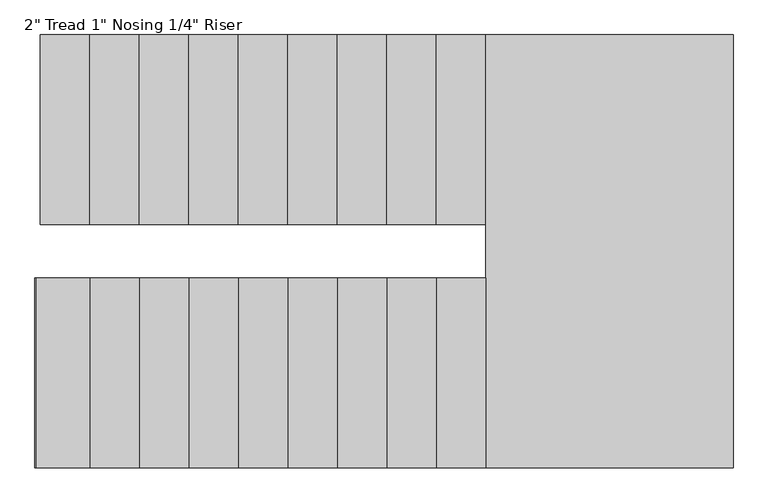
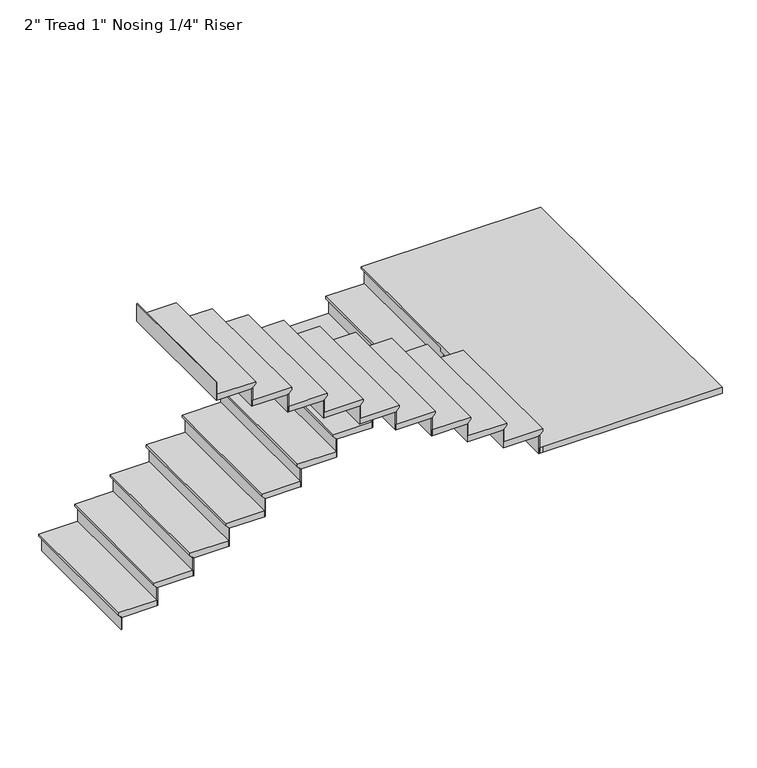
"""IFC4 building model written with IfcOpenShell, lengths in millimetres: stair flight geometry."""

from ifc_helpers import new_model, si_unit, origin, place, context, project, spatial, faceted_brep, source, transform, mapped, element, save


def stair_flight_54cbe99c(model_context):
    return source(origin(), model_context, "Body", "Brep", [
        faceted_brep([(9166.2546318, 21751.034892, 140.97), (9166.2546318, 21751.034892, 160.02), (9166.2546318, 22919.434892, 160.02), (9166.2546318, 22919.434892, 140.97), (9191.6546318, 21751.034892, 115.57), (9191.6546318, 22919.434892, 115.57), (9496.4546318, 21751.034892, 160.02), (9496.4546318, 22919.434892, 160.02), (9191.6546318, 22919.434892, 109.22), (9496.4546318, 22919.434892, 109.22), (9496.4546318, 21751.034892, 109.22), (9191.6546318, 21751.034892, 109.22)], [[[0, 1, 2, 3]], [[4, 0, 3, 5]], [[2, 1, 6, 7]], [[8, 9, 10, 11]], [[2, 7, 9, 8, 5, 3]], [[8, 11, 4, 5]], [[6, 1, 0, 4, 11, 10]], [[7, 6, 10, 9]]]),
        faceted_brep([(9191.6546318, 21751.034892, 109.22), (9191.6546318, 21751.034892, 0.0), (9198.0046318, 21751.034892, 0.0), (9198.0046318, 21751.034892, 109.22), (9191.6546318, 22919.434892, 109.22), (9198.0046318, 22919.434892, 109.22), (9198.0046318, 22919.434892, 0.0), (9191.6546318, 22919.434892, 0.0)], [[[0, 1, 2, 3]], [[4, 5, 6, 7]], [[1, 0, 4, 7]], [[2, 1, 7, 6]], [[3, 2, 6, 5]], [[0, 3, 5, 4]]]),
        faceted_brep([(9496.4546318, 21751.034892, 269.24), (9496.4546318, 21751.034892, 109.22), (9502.8046318, 21751.034892, 109.22), (9502.8046318, 21751.034892, 269.24), (9496.4546318, 22919.434892, 269.24), (9502.8046318, 22919.434892, 269.24), (9502.8046318, 22919.434892, 109.22), (9496.4546318, 22919.434892, 109.22)], [[[0, 1, 2, 3]], [[4, 5, 6, 7]], [[1, 0, 4, 7]], [[2, 1, 7, 6]], [[3, 2, 6, 5]], [[0, 3, 5, 4]]]),
        faceted_brep([(9471.0546318, 22919.434892, 320.04), (9471.0546318, 21751.034892, 320.04), (9801.2546318, 21751.034892, 320.04), (9801.2546318, 22919.434892, 320.04), (9496.4546318, 22919.434892, 269.24), (9801.2546318, 22919.434892, 269.24), (9801.2546318, 21751.034892, 269.24), (9496.4546318, 21751.034892, 269.24), (9496.4546318, 22919.434892, 275.59), (9471.0546318, 22919.434892, 300.99), (9496.4546318, 21751.034892, 275.59), (9471.0546318, 21751.034892, 300.99)], [[[0, 1, 2, 3]], [[4, 5, 6, 7]], [[0, 3, 5, 4, 8, 9]], [[4, 7, 10, 8]], [[2, 1, 11, 10, 7, 6]], [[3, 2, 6, 5]], [[11, 1, 0, 9]], [[10, 11, 9, 8]]]),
        faceted_brep([(9801.2546318, 21751.034892, 429.26), (9801.2546318, 21751.034892, 269.24), (9807.6046318, 21751.034892, 269.24), (9807.6046318, 21751.034892, 429.26), (9801.2546318, 22919.434892, 429.26), (9807.6046318, 22919.434892, 429.26), (9807.6046318, 22919.434892, 269.24), (9801.2546318, 22919.434892, 269.24)], [[[0, 1, 2, 3]], [[4, 5, 6, 7]], [[1, 0, 4, 7]], [[2, 1, 7, 6]], [[3, 2, 6, 5]], [[0, 3, 5, 4]]]),
        faceted_brep([(9775.8546318, 22919.434892, 480.06), (9775.8546318, 21751.034892, 480.06), (10106.0546318, 21751.034892, 480.06), (10106.0546318, 22919.434892, 480.06), (9801.2546318, 22919.434892, 429.26), (10106.0546318, 22919.434892, 429.26), (10106.0546318, 21751.034892, 429.26), (9801.2546318, 21751.034892, 429.26), (9801.2546318, 22919.434892, 435.61), (9775.8546318, 22919.434892, 461.01), (9801.2546318, 21751.034892, 435.61), (9775.8546318, 21751.034892, 461.01)], [[[0, 1, 2, 3]], [[4, 5, 6, 7]], [[0, 3, 5, 4, 8, 9]], [[4, 7, 10, 8]], [[2, 1, 11, 10, 7, 6]], [[3, 2, 6, 5]], [[11, 1, 0, 9]], [[10, 11, 9, 8]]]),
        faceted_brep([(10106.0546318, 21751.034892, 589.28), (10106.0546318, 21751.034892, 429.26), (10112.4046318, 21751.034892, 429.26), (10112.4046318, 21751.034892, 589.28), (10106.0546318, 22919.434892, 589.28), (10112.4046318, 22919.434892, 589.28), (10112.4046318, 22919.434892, 429.26), (10106.0546318, 22919.434892, 429.26)], [[[0, 1, 2, 3]], [[4, 5, 6, 7]], [[1, 0, 4, 7]], [[2, 1, 7, 6]], [[3, 2, 6, 5]], [[0, 3, 5, 4]]]),
        faceted_brep([(10080.6546318, 22919.434892, 640.08), (10080.6546318, 21751.034892, 640.08), (10410.8546318, 21751.034892, 640.08), (10410.8546318, 22919.434892, 640.08), (10106.0546318, 22919.434892, 589.28), (10410.8546318, 22919.434892, 589.28), (10410.8546318, 21751.034892, 589.28), (10106.0546318, 21751.034892, 589.28), (10106.0546318, 22919.434892, 595.63), (10080.6546318, 22919.434892, 621.03), (10106.0546318, 21751.034892, 595.63), (10080.6546318, 21751.034892, 621.03)], [[[0, 1, 2, 3]], [[4, 5, 6, 7]], [[0, 3, 5, 4, 8, 9]], [[4, 7, 10, 8]], [[2, 1, 11, 10, 7, 6]], [[3, 2, 6, 5]], [[11, 1, 0, 9]], [[10, 11, 9, 8]]]),
        faceted_brep([(10410.8546318, 21751.034892, 749.3), (10410.8546318, 21751.034892, 589.28), (10417.2046318, 21751.034892, 589.28), (10417.2046318, 21751.034892, 749.3), (10410.8546318, 22919.434892, 749.3), (10417.2046318, 22919.434892, 749.3), (10417.2046318, 22919.434892, 589.28), (10410.8546318, 22919.434892, 589.28)], [[[0, 1, 2, 3]], [[4, 5, 6, 7]], [[1, 0, 4, 7]], [[2, 1, 7, 6]], [[3, 2, 6, 5]], [[0, 3, 5, 4]]]),
        faceted_brep([(10385.4546318, 22919.434892, 800.1), (10385.4546318, 21751.034892, 800.1), (10715.6546318, 21751.034892, 800.1), (10715.6546318, 22919.434892, 800.1), (10410.8546318, 22919.434892, 749.3), (10715.6546318, 22919.434892, 749.3), (10715.6546318, 21751.034892, 749.3), (10410.8546318, 21751.034892, 749.3), (10410.8546318, 22919.434892, 755.65), (10385.4546318, 22919.434892, 781.05), (10410.8546318, 21751.034892, 755.65), (10385.4546318, 21751.034892, 781.05)], [[[0, 1, 2, 3]], [[4, 5, 6, 7]], [[0, 3, 5, 4, 8, 9]], [[4, 7, 10, 8]], [[2, 1, 11, 10, 7, 6]], [[3, 2, 6, 5]], [[11, 1, 0, 9]], [[10, 11, 9, 8]]]),
        faceted_brep([(10715.6546318, 21751.034892, 909.32), (10715.6546318, 21751.034892, 749.3), (10722.0046318, 21751.034892, 749.3), (10722.0046318, 21751.034892, 909.32), (10715.6546318, 22919.434892, 909.32), (10722.0046318, 22919.434892, 909.32), (10722.0046318, 22919.434892, 749.3), (10715.6546318, 22919.434892, 749.3)], [[[0, 1, 2, 3]], [[4, 5, 6, 7]], [[1, 0, 4, 7]], [[2, 1, 7, 6]], [[3, 2, 6, 5]], [[0, 3, 5, 4]]]),
        faceted_brep([(10690.2546318, 22919.434892, 960.12), (10690.2546318, 21751.034892, 960.12), (11020.4546318, 21751.034892, 960.12), (11020.4546318, 22919.434892, 960.12), (10715.6546318, 22919.434892, 909.32), (11020.4546318, 22919.434892, 909.32), (11020.4546318, 21751.034892, 909.32), (10715.6546318, 21751.034892, 909.32), (10715.6546318, 22919.434892, 915.67), (10690.2546318, 22919.434892, 941.07), (10715.6546318, 21751.034892, 915.67), (10690.2546318, 21751.034892, 941.07)], [[[0, 1, 2, 3]], [[4, 5, 6, 7]], [[0, 3, 5, 4, 8, 9]], [[4, 7, 10, 8]], [[2, 1, 11, 10, 7, 6]], [[3, 2, 6, 5]], [[11, 1, 0, 9]], [[10, 11, 9, 8]]]),
        faceted_brep([(11020.4546318, 21751.034892, 1069.34), (11020.4546318, 21751.034892, 909.32), (11026.8046318, 21751.034892, 909.32), (11026.8046318, 21751.034892, 1069.34), (11020.4546318, 22919.434892, 1069.34), (11026.8046318, 22919.434892, 1069.34), (11026.8046318, 22919.434892, 909.32), (11020.4546318, 22919.434892, 909.32)], [[[0, 1, 2, 3]], [[4, 5, 6, 7]], [[1, 0, 4, 7]], [[2, 1, 7, 6]], [[3, 2, 6, 5]], [[0, 3, 5, 4]]]),
        faceted_brep([(10995.0546318, 22919.434892, 1120.14), (10995.0546318, 21751.034892, 1120.14), (11325.2546318, 21751.034892, 1120.14), (11325.2546318, 22919.434892, 1120.14), (11020.4546318, 22919.434892, 1069.34), (11325.2546318, 22919.434892, 1069.34), (11325.2546318, 21751.034892, 1069.34), (11020.4546318, 21751.034892, 1069.34), (11020.4546318, 22919.434892, 1075.69), (10995.0546318, 22919.434892, 1101.09), (11020.4546318, 21751.034892, 1075.69), (10995.0546318, 21751.034892, 1101.09)], [[[0, 1, 2, 3]], [[4, 5, 6, 7]], [[0, 3, 5, 4, 8, 9]], [[4, 7, 10, 8]], [[2, 1, 11, 10, 7, 6]], [[3, 2, 6, 5]], [[11, 1, 0, 9]], [[10, 11, 9, 8]]]),
        faceted_brep([(11325.2546318, 21751.034892, 1229.36), (11325.2546318, 21751.034892, 1069.34), (11331.6046318, 21751.034892, 1069.34), (11331.6046318, 21751.034892, 1229.36), (11325.2546318, 22919.434892, 1229.36), (11331.6046318, 22919.434892, 1229.36), (11331.6046318, 22919.434892, 1069.34), (11325.2546318, 22919.434892, 1069.34)], [[[0, 1, 2, 3]], [[4, 5, 6, 7]], [[1, 0, 4, 7]], [[2, 1, 7, 6]], [[3, 2, 6, 5]], [[0, 3, 5, 4]]]),
        faceted_brep([(11299.8546318, 22919.434892, 1280.16), (11299.8546318, 21751.034892, 1280.16), (11630.0546318, 21751.034892, 1280.16), (11630.0546318, 22919.434892, 1280.16), (11325.2546318, 22919.434892, 1229.36), (11630.0546318, 22919.434892, 1229.36), (11630.0546318, 21751.034892, 1229.36), (11325.2546318, 21751.034892, 1229.36), (11325.2546318, 22919.434892, 1235.71), (11299.8546318, 22919.434892, 1261.11), (11325.2546318, 21751.034892, 1235.71), (11299.8546318, 21751.034892, 1261.11)], [[[0, 1, 2, 3]], [[4, 5, 6, 7]], [[0, 3, 5, 4, 8, 9]], [[4, 7, 10, 8]], [[2, 1, 11, 10, 7, 6]], [[3, 2, 6, 5]], [[11, 1, 0, 9]], [[10, 11, 9, 8]]]),
        faceted_brep([(11630.0546318, 21751.034892, 1389.38), (11630.0546318, 21751.034892, 1229.36), (11636.4046318, 21751.034892, 1229.36), (11636.4046318, 21751.034892, 1389.38), (11630.0546318, 22919.434892, 1389.38), (11636.4046318, 22919.434892, 1389.38), (11636.4046318, 22919.434892, 1229.36), (11630.0546318, 22919.434892, 1229.36)], [[[0, 1, 2, 3]], [[4, 5, 6, 7]], [[1, 0, 4, 7]], [[2, 1, 7, 6]], [[3, 2, 6, 5]], [[0, 3, 5, 4]]]),
        faceted_brep([(11604.6546318, 22919.434892, 1440.18), (11604.6546318, 21751.034892, 1440.18), (11934.8546318, 21751.034892, 1440.18), (11934.8546318, 22919.434892, 1440.18), (11630.0546318, 22919.434892, 1389.38), (11934.8546318, 22919.434892, 1389.38), (11934.8546318, 21751.034892, 1389.38), (11630.0546318, 21751.034892, 1389.38), (11630.0546318, 22919.434892, 1395.73), (11604.6546318, 22919.434892, 1421.13), (11630.0546318, 21751.034892, 1395.73), (11604.6546318, 21751.034892, 1421.13)], [[[0, 1, 2, 3]], [[4, 5, 6, 7]], [[0, 3, 5, 4, 8, 9]], [[4, 7, 10, 8]], [[2, 1, 11, 10, 7, 6]], [[3, 2, 6, 5]], [[11, 1, 0, 9]], [[10, 11, 9, 8]]]),
        faceted_brep([(11934.8546318, 21751.034892, 1549.4), (11934.8546318, 21751.034892, 1389.38), (11941.2046318, 21751.034892, 1389.38), (11941.2046318, 21751.034892, 1549.4), (11934.8546318, 22919.434892, 1549.4), (11941.2046318, 22919.434892, 1549.4), (11941.2046318, 22919.434892, 1389.38), (11934.8546318, 22919.434892, 1389.38)], [[[0, 1, 2, 3]], [[4, 5, 6, 7]], [[1, 0, 4, 7]], [[2, 1, 7, 6]], [[3, 2, 6, 5]], [[0, 3, 5, 4]]]),
        faceted_brep([(11884.0546318, 20252.434892, 1600.2), (11909.4546318, 20252.434892, 1600.2), (13433.4546318, 20252.434892, 1600.2), (13433.4546318, 22919.434892, 1600.2), (11909.4546318, 22919.434892, 1600.2), (11909.4546318, 21420.834892, 1600.2), (11884.0546318, 21420.834892, 1600.2), (11909.4546318, 20252.434892, 1549.4), (11884.0546318, 20252.434892, 1549.4), (11884.0546318, 21420.834892, 1549.4), (11909.4546318, 21420.834892, 1549.4), (11909.4546318, 21751.034892, 1549.4), (11934.8546318, 21751.034892, 1549.4), (11934.8546318, 22919.434892, 1549.4), (13433.4546318, 22919.434892, 1549.4), (13433.4546318, 20252.434892, 1549.4), (11934.8546318, 22919.434892, 1555.75), (11909.4546318, 22919.434892, 1581.15), (11934.8546318, 21751.034892, 1555.75), (11909.4546318, 21751.034892, 1581.15)], [[[0, 1, 2, 3, 4, 5, 6]], [[7, 8, 9, 10, 11, 12, 13, 14, 15]], [[1, 0, 8, 7]], [[2, 1, 7, 15]], [[3, 2, 15, 14]], [[4, 3, 14, 13, 16, 17]], [[13, 12, 18, 16]], [[12, 11, 19, 18]], [[5, 4, 17, 19, 11, 10]], [[6, 5, 10, 9]], [[0, 6, 9, 8]], [[17, 16, 18, 19]]]),
        faceted_brep([(11884.0546318, 21420.834892, 1709.42), (11884.0546318, 21420.834892, 1549.4), (11877.7046318, 21420.834892, 1549.4), (11877.7046318, 21420.834892, 1709.42), (11884.0546318, 20252.434892, 1709.42), (11877.7046318, 20252.434892, 1709.42), (11877.7046318, 20252.434892, 1549.4), (11884.0546318, 20252.434892, 1549.4)], [[[0, 1, 2, 3]], [[4, 5, 6, 7]], [[1, 0, 4, 7]], [[2, 1, 7, 6]], [[3, 2, 6, 5]], [[0, 3, 5, 4]]]),
        faceted_brep([(11909.4546318, 20252.434892, 1760.22), (11909.4546318, 21420.834892, 1760.22), (11579.2546318, 21420.834892, 1760.22), (11579.2546318, 20252.434892, 1760.22), (11884.0546318, 20252.434892, 1709.42), (11579.2546318, 20252.434892, 1709.42), (11579.2546318, 21420.834892, 1709.42), (11884.0546318, 21420.834892, 1709.42), (11884.0546318, 20252.434892, 1715.77), (11909.4546318, 20252.434892, 1741.17), (11884.0546318, 21420.834892, 1715.77), (11909.4546318, 21420.834892, 1741.17)], [[[0, 1, 2, 3]], [[4, 5, 6, 7]], [[0, 3, 5, 4, 8, 9]], [[4, 7, 10, 8]], [[2, 1, 11, 10, 7, 6]], [[3, 2, 6, 5]], [[11, 1, 0, 9]], [[10, 11, 9, 8]]]),
        faceted_brep([(11579.2546318, 21420.834892, 1869.44), (11579.2546318, 21420.834892, 1709.42), (11572.9046318, 21420.834892, 1709.42), (11572.9046318, 21420.834892, 1869.44), (11579.2546318, 20252.434892, 1869.44), (11572.9046318, 20252.434892, 1869.44), (11572.9046318, 20252.434892, 1709.42), (11579.2546318, 20252.434892, 1709.42)], [[[0, 1, 2, 3]], [[4, 5, 6, 7]], [[1, 0, 4, 7]], [[2, 1, 7, 6]], [[3, 2, 6, 5]], [[0, 3, 5, 4]]]),
        faceted_brep([(11604.6546318, 20252.434892, 1920.24), (11604.6546318, 21420.834892, 1920.24), (11274.4546318, 21420.834892, 1920.24), (11274.4546318, 20252.434892, 1920.24), (11579.2546318, 20252.434892, 1869.44), (11274.4546318, 20252.434892, 1869.44), (11274.4546318, 21420.834892, 1869.44), (11579.2546318, 21420.834892, 1869.44), (11579.2546318, 20252.434892, 1875.79), (11604.6546318, 20252.434892, 1901.19), (11579.2546318, 21420.834892, 1875.79), (11604.6546318, 21420.834892, 1901.19)], [[[0, 1, 2, 3]], [[4, 5, 6, 7]], [[0, 3, 5, 4, 8, 9]], [[4, 7, 10, 8]], [[2, 1, 11, 10, 7, 6]], [[3, 2, 6, 5]], [[11, 1, 0, 9]], [[10, 11, 9, 8]]]),
        faceted_brep([(11274.4546318, 21420.834892, 2029.46), (11274.4546318, 21420.834892, 1869.44), (11268.1046318, 21420.834892, 1869.44), (11268.1046318, 21420.834892, 2029.46), (11274.4546318, 20252.434892, 2029.46), (11268.1046318, 20252.434892, 2029.46), (11268.1046318, 20252.434892, 1869.44), (11274.4546318, 20252.434892, 1869.44)], [[[0, 1, 2, 3]], [[4, 5, 6, 7]], [[1, 0, 4, 7]], [[2, 1, 7, 6]], [[3, 2, 6, 5]], [[0, 3, 5, 4]]]),
        faceted_brep([(11299.8546318, 20252.434892, 2080.26), (11299.8546318, 21420.834892, 2080.26), (10969.6546318, 21420.834892, 2080.26), (10969.6546318, 20252.434892, 2080.26), (11274.4546318, 20252.434892, 2029.46), (10969.6546318, 20252.434892, 2029.46), (10969.6546318, 21420.834892, 2029.46), (11274.4546318, 21420.834892, 2029.46), (11274.4546318, 20252.434892, 2035.81), (11299.8546318, 20252.434892, 2061.21), (11274.4546318, 21420.834892, 2035.81), (11299.8546318, 21420.834892, 2061.21)], [[[0, 1, 2, 3]], [[4, 5, 6, 7]], [[0, 3, 5, 4, 8, 9]], [[4, 7, 10, 8]], [[2, 1, 11, 10, 7, 6]], [[3, 2, 6, 5]], [[11, 1, 0, 9]], [[10, 11, 9, 8]]]),
        faceted_brep([(10969.6546318, 21420.834892, 2189.48), (10969.6546318, 21420.834892, 2029.46), (10963.3046318, 21420.834892, 2029.46), (10963.3046318, 21420.834892, 2189.48), (10969.6546318, 20252.434892, 2189.48), (10963.3046318, 20252.434892, 2189.48), (10963.3046318, 20252.434892, 2029.46), (10969.6546318, 20252.434892, 2029.46)], [[[0, 1, 2, 3]], [[4, 5, 6, 7]], [[1, 0, 4, 7]], [[2, 1, 7, 6]], [[3, 2, 6, 5]], [[0, 3, 5, 4]]]),
        faceted_brep([(10995.0546318, 20252.434892, 2240.28), (10995.0546318, 21420.834892, 2240.28), (10664.8546318, 21420.834892, 2240.28), (10664.8546318, 20252.434892, 2240.28), (10969.6546318, 20252.434892, 2189.48), (10664.8546318, 20252.434892, 2189.48), (10664.8546318, 21420.834892, 2189.48), (10969.6546318, 21420.834892, 2189.48), (10969.6546318, 20252.434892, 2195.83), (10995.0546318, 20252.434892, 2221.23), (10969.6546318, 21420.834892, 2195.83), (10995.0546318, 21420.834892, 2221.23)], [[[0, 1, 2, 3]], [[4, 5, 6, 7]], [[0, 3, 5, 4, 8, 9]], [[4, 7, 10, 8]], [[2, 1, 11, 10, 7, 6]], [[3, 2, 6, 5]], [[11, 1, 0, 9]], [[10, 11, 9, 8]]]),
        faceted_brep([(10664.8546318, 21420.834892, 2349.5), (10664.8546318, 21420.834892, 2189.48), (10658.5046318, 21420.834892, 2189.48), (10658.5046318, 21420.834892, 2349.5), (10664.8546318, 20252.434892, 2349.5), (10658.5046318, 20252.434892, 2349.5), (10658.5046318, 20252.434892, 2189.48), (10664.8546318, 20252.434892, 2189.48)], [[[0, 1, 2, 3]], [[4, 5, 6, 7]], [[1, 0, 4, 7]], [[2, 1, 7, 6]], [[3, 2, 6, 5]], [[0, 3, 5, 4]]]),
        faceted_brep([(10690.2546318, 20252.434892, 2400.3), (10690.2546318, 21420.834892, 2400.3), (10360.0546318, 21420.834892, 2400.3), (10360.0546318, 20252.434892, 2400.3), (10664.8546318, 20252.434892, 2349.5), (10360.0546318, 20252.434892, 2349.5), (10360.0546318, 21420.834892, 2349.5), (10664.8546318, 21420.834892, 2349.5), (10664.8546318, 20252.434892, 2355.85), (10690.2546318, 20252.434892, 2381.25), (10664.8546318, 21420.834892, 2355.85), (10690.2546318, 21420.834892, 2381.25)], [[[0, 1, 2, 3]], [[4, 5, 6, 7]], [[0, 3, 5, 4, 8, 9]], [[4, 7, 10, 8]], [[2, 1, 11, 10, 7, 6]], [[3, 2, 6, 5]], [[11, 1, 0, 9]], [[10, 11, 9, 8]]]),
        faceted_brep([(10360.0546318, 21420.834892, 2509.52), (10360.0546318, 21420.834892, 2349.5), (10353.7046318, 21420.834892, 2349.5), (10353.7046318, 21420.834892, 2509.52), (10360.0546318, 20252.434892, 2509.52), (10353.7046318, 20252.434892, 2509.52), (10353.7046318, 20252.434892, 2349.5), (10360.0546318, 20252.434892, 2349.5)], [[[0, 1, 2, 3]], [[4, 5, 6, 7]], [[1, 0, 4, 7]], [[2, 1, 7, 6]], [[3, 2, 6, 5]], [[0, 3, 5, 4]]]),
        faceted_brep([(10385.4546318, 20252.434892, 2560.32), (10385.4546318, 21420.834892, 2560.32), (10055.2546318, 21420.834892, 2560.32), (10055.2546318, 20252.434892, 2560.32), (10360.0546318, 20252.434892, 2509.52), (10055.2546318, 20252.434892, 2509.52), (10055.2546318, 21420.834892, 2509.52), (10360.0546318, 21420.834892, 2509.52), (10360.0546318, 20252.434892, 2515.87), (10385.4546318, 20252.434892, 2541.27), (10360.0546318, 21420.834892, 2515.87), (10385.4546318, 21420.834892, 2541.27)], [[[0, 1, 2, 3]], [[4, 5, 6, 7]], [[0, 3, 5, 4, 8, 9]], [[4, 7, 10, 8]], [[2, 1, 11, 10, 7, 6]], [[3, 2, 6, 5]], [[11, 1, 0, 9]], [[10, 11, 9, 8]]]),
        faceted_brep([(10055.2546318, 21420.834892, 2669.54), (10055.2546318, 21420.834892, 2509.52), (10048.9046318, 21420.834892, 2509.52), (10048.9046318, 21420.834892, 2669.54), (10055.2546318, 20252.434892, 2669.54), (10048.9046318, 20252.434892, 2669.54), (10048.9046318, 20252.434892, 2509.52), (10055.2546318, 20252.434892, 2509.52)], [[[0, 1, 2, 3]], [[4, 5, 6, 7]], [[1, 0, 4, 7]], [[2, 1, 7, 6]], [[3, 2, 6, 5]], [[0, 3, 5, 4]]]),
        faceted_brep([(10080.6546318, 20252.434892, 2720.34), (10080.6546318, 21420.834892, 2720.34), (9750.4546318, 21420.834892, 2720.34), (9750.4546318, 20252.434892, 2720.34), (10055.2546318, 20252.434892, 2669.54), (9750.4546318, 20252.434892, 2669.54), (9750.4546318, 21420.834892, 2669.54), (10055.2546318, 21420.834892, 2669.54), (10055.2546318, 20252.434892, 2675.89), (10080.6546318, 20252.434892, 2701.29), (10055.2546318, 21420.834892, 2675.89), (10080.6546318, 21420.834892, 2701.29)], [[[0, 1, 2, 3]], [[4, 5, 6, 7]], [[0, 3, 5, 4, 8, 9]], [[4, 7, 10, 8]], [[2, 1, 11, 10, 7, 6]], [[3, 2, 6, 5]], [[11, 1, 0, 9]], [[10, 11, 9, 8]]]),
        faceted_brep([(9750.4546318, 21420.834892, 2829.56), (9750.4546318, 21420.834892, 2669.54), (9744.1046318, 21420.834892, 2669.54), (9744.1046318, 21420.834892, 2829.56), (9750.4546318, 20252.434892, 2829.56), (9744.1046318, 20252.434892, 2829.56), (9744.1046318, 20252.434892, 2669.54), (9750.4546318, 20252.434892, 2669.54)], [[[0, 1, 2, 3]], [[4, 5, 6, 7]], [[1, 0, 4, 7]], [[2, 1, 7, 6]], [[3, 2, 6, 5]], [[0, 3, 5, 4]]]),
        faceted_brep([(9775.8546318, 20252.434892, 2880.36), (9775.8546318, 21420.834892, 2880.36), (9445.6546318, 21420.834892, 2880.36), (9445.6546318, 20252.434892, 2880.36), (9750.4546318, 20252.434892, 2829.56), (9445.6546318, 20252.434892, 2829.56), (9445.6546318, 21420.834892, 2829.56), (9750.4546318, 21420.834892, 2829.56), (9750.4546318, 20252.434892, 2835.91), (9775.8546318, 20252.434892, 2861.31), (9750.4546318, 21420.834892, 2835.91), (9775.8546318, 21420.834892, 2861.31)], [[[0, 1, 2, 3]], [[4, 5, 6, 7]], [[0, 3, 5, 4, 8, 9]], [[4, 7, 10, 8]], [[2, 1, 11, 10, 7, 6]], [[3, 2, 6, 5]], [[11, 1, 0, 9]], [[10, 11, 9, 8]]]),
        faceted_brep([(9445.6546318, 21420.834892, 2989.58), (9445.6546318, 21420.834892, 2829.56), (9439.3046318, 21420.834892, 2829.56), (9439.3046318, 21420.834892, 2989.58), (9445.6546318, 20252.434892, 2989.58), (9439.3046318, 20252.434892, 2989.58), (9439.3046318, 20252.434892, 2829.56), (9445.6546318, 20252.434892, 2829.56)], [[[0, 1, 2, 3]], [[4, 5, 6, 7]], [[1, 0, 4, 7]], [[2, 1, 7, 6]], [[3, 2, 6, 5]], [[0, 3, 5, 4]]]),
        faceted_brep([(9140.8546318, 21420.834892, 3149.6), (9140.8546318, 21420.834892, 2989.58), (9134.5046318, 21420.834892, 2989.58), (9134.5046318, 21420.834892, 3149.6), (9140.8546318, 20252.434892, 3149.6), (9134.5046318, 20252.434892, 3149.6), (9134.5046318, 20252.434892, 2989.58), (9140.8546318, 20252.434892, 2989.58)], [[[0, 1, 2, 3]], [[4, 5, 6, 7]], [[1, 0, 4, 7]], [[2, 1, 7, 6]], [[3, 2, 6, 5]], [[0, 3, 5, 4]]]),
        faceted_brep([(9471.0546318, 20252.434892, 3040.38), (9471.0546318, 21420.834892, 3040.38), (9140.8546318, 21420.834892, 3040.38), (9140.8546318, 20252.434892, 3040.38), (9445.6546318, 20252.434892, 2989.58), (9140.8546318, 20252.434892, 2989.58), (9140.8546318, 21420.834892, 2989.58), (9445.6546318, 21420.834892, 2989.58), (9445.6546318, 20252.434892, 2995.93), (9471.0546318, 20252.434892, 3021.33), (9445.6546318, 21420.834892, 2995.93), (9471.0546318, 21420.834892, 3021.33)], [[[0, 1, 2, 3]], [[4, 5, 6, 7]], [[0, 3, 5, 4, 8, 9]], [[4, 7, 10, 8]], [[2, 1, 11, 10, 7, 6]], [[3, 2, 6, 5]], [[11, 1, 0, 9]], [[10, 11, 9, 8]]]),
    ])


if __name__ == "__main__":
    model = new_model("IFC4")
    model_context = context("Model", 3, world=origin())
    ifc_project = project(units=[si_unit("LENGTHUNIT", "METRE", prefix="MILLI")], contexts=[model_context])
    site = spatial("IfcSite", under=ifc_project)
    building = spatial("IfcBuilding", under=site)
    placement = place(None, origin())
    stair_flight_shape = stair_flight_54cbe99c(model_context)
    element("IfcStairFlight", 1, ObjectType="2\" Tread 1\" Nosing 1/4\" Riser", at=placement, inside=building, context=model_context, shape_type="MappedRepresentation", body=[
        mapped(stair_flight_shape, transform((0.0, 0.0, 0.0), x_axis=(1.0, 0.0, 0.0), y_axis=(0.0, 1.0, 0.0), z_axis=(0.0, 0.0, 1.0))),
    ])
    save(model, "model.ifc")
